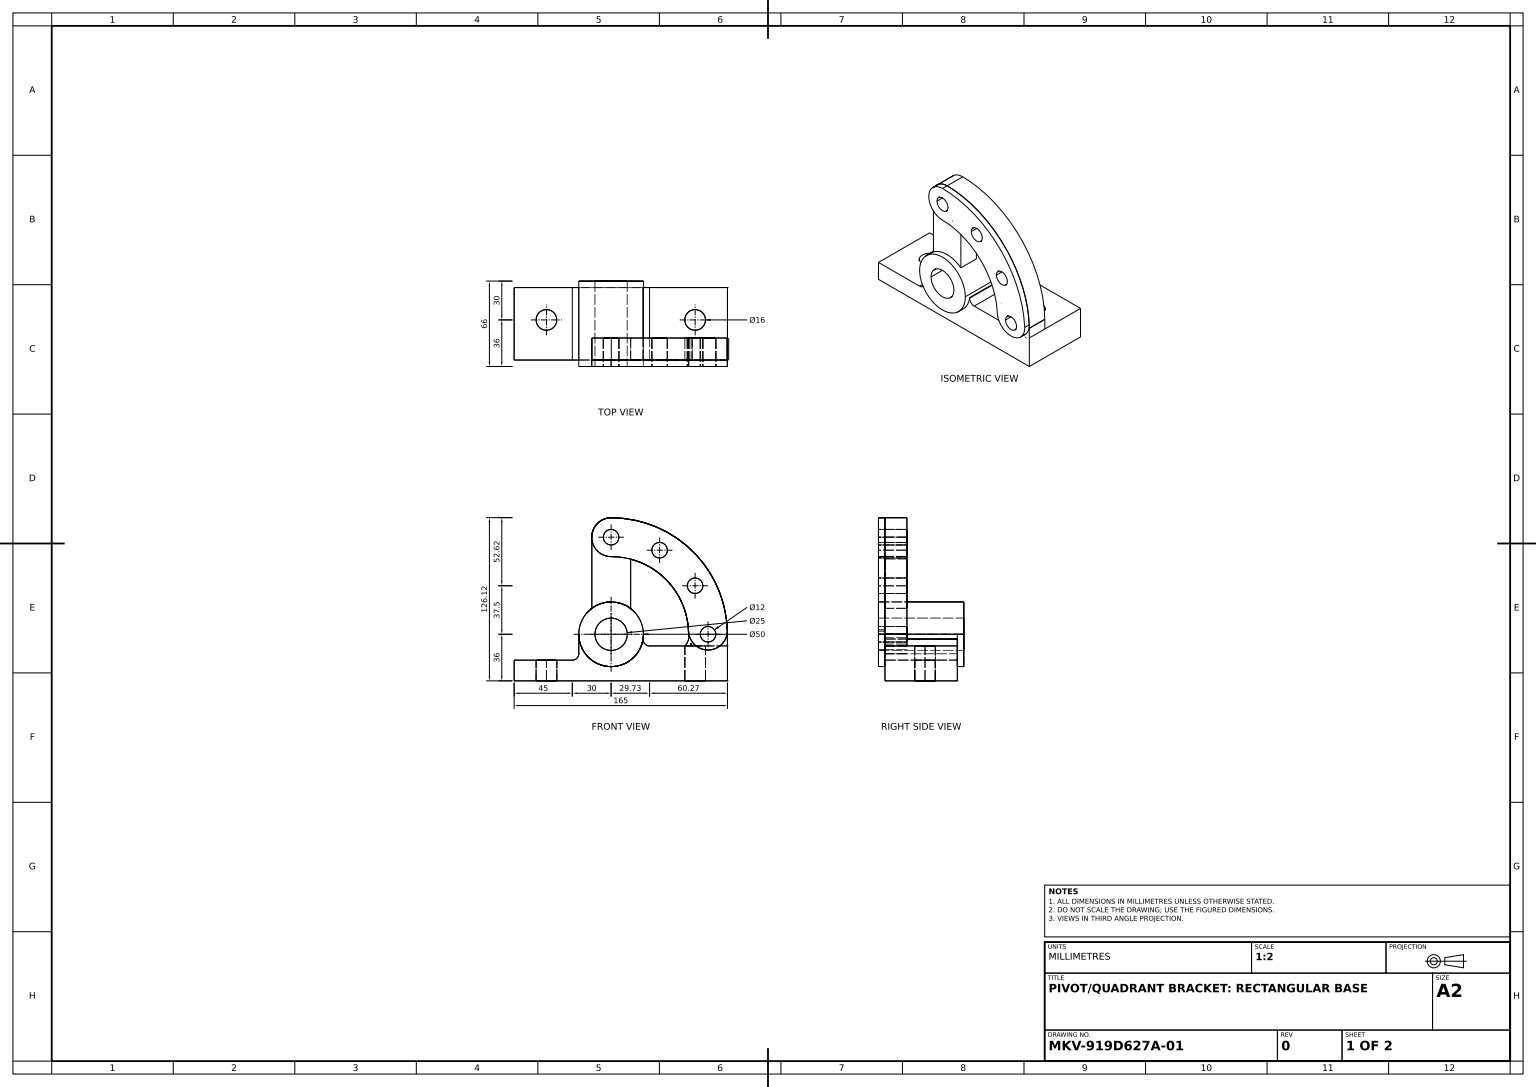
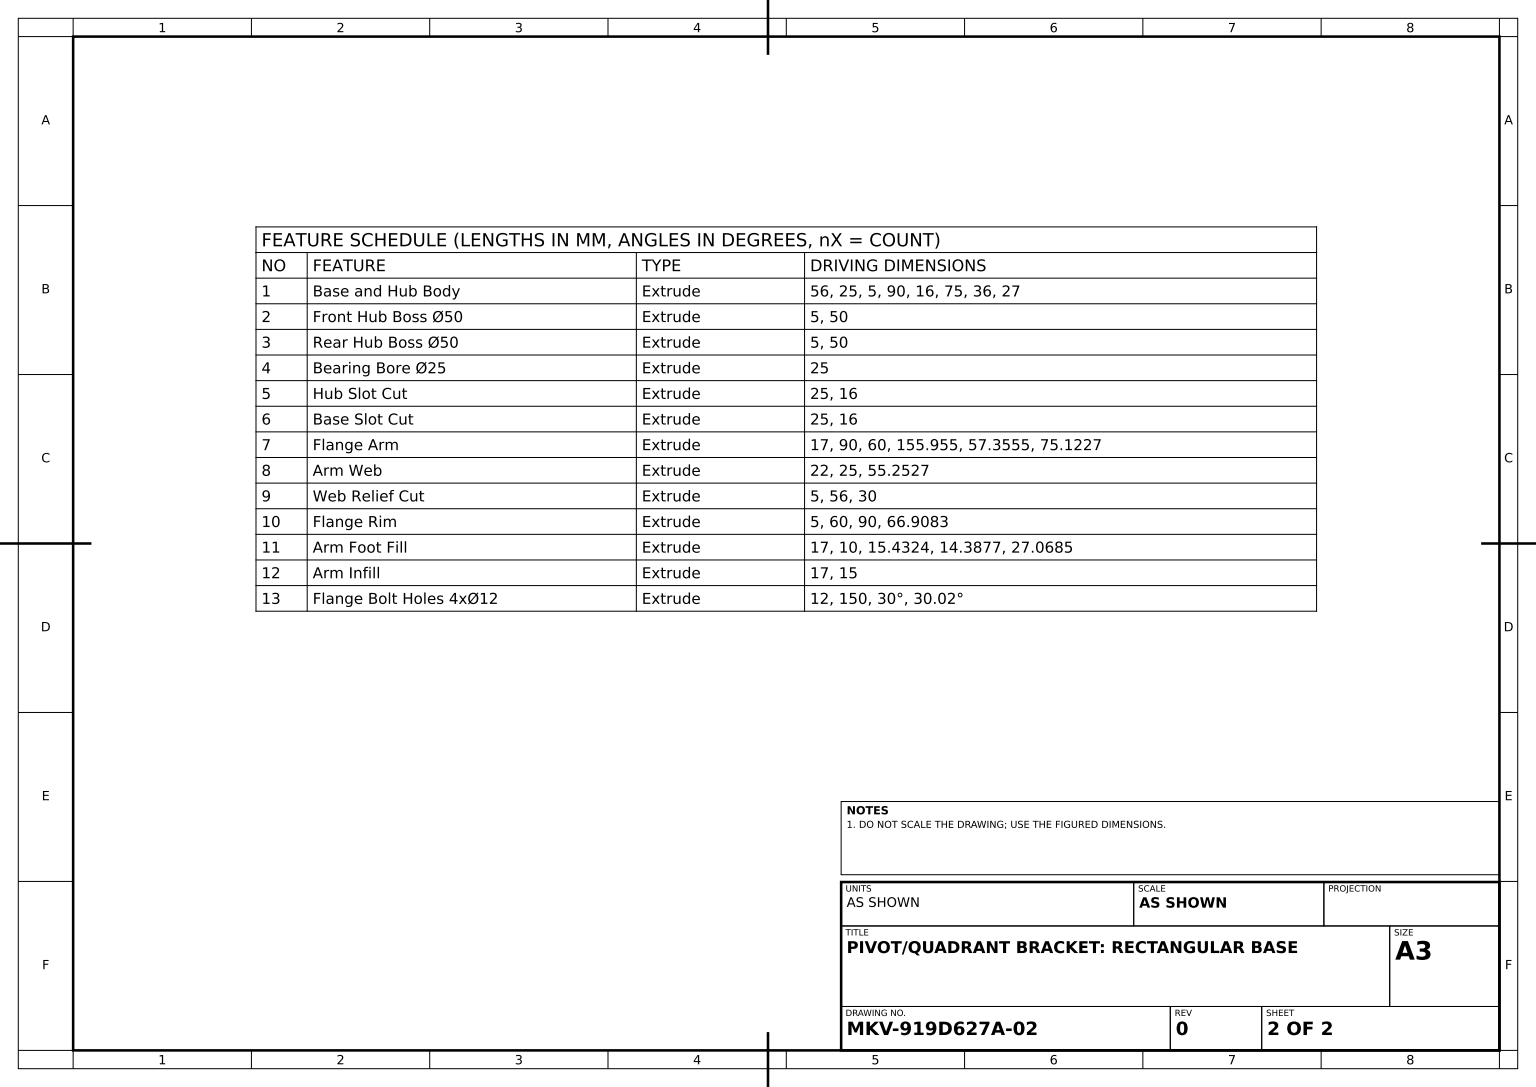
SolidWorks part; units mm, degrees
material "Plain Carbon Steel"
ref_plane "Front Plane" through (0, 0, 0) normal (0, 0, 1) x (1, 0, 0)
ref_plane "Top Plane" through (0, 0, 0) normal (0, 1, 0) x (1, 0, 0)
ref_plane "Right Plane" through (0, 0, 0) normal (1, 0, 0) x (0, 0, -1)
sketch "Base and Hub Profile Sketch" plane through (0, 0, 0) normal (0, 0, 1) x (1, 0, 0)
  line L0 (0, 0) -> (165, 0)
  line L1 (165, 0) -> (165, 27)
  line L2 (165, 27) -> (104.7321, 27)
  line L3 (0, 0) -> (0, 16)
  line L4 (0, 16) -> (45, 16)
  line L9 (50, 36) -> (50, 21)
  arc A0 (99.7768, 32.6667) -> (50, 36) centre (75, 36) ccw
  arc A1 (45, 16) -> (50, 21) centre (45, 21) ccw
  arc A2 (99.7768, 32.6667) -> (104.7321, 27) centre (104.7321, 32) ccw
  dimension "D1" = 75
  dimension "D2" = 25
  dimension "D4" = 5
  dimension "D8" = 5
  dimension "D3" = 36
  dimension "D5" = 90
  dimension "D6" = 16
  dimension "D7" = 27
extrude "Base and Hub Body" add sketch "Base and Hub Profile Sketch" along normal mid plane 56
sketch "Front Hub Boss Sketch" plane through (0, 0, 28) normal (0, 0, 1) x (1, 0, 0)
  circle A0 centre (75, 36) radius 25
  dimension "D1" = 50
extrude "Front Hub Boss Ø50" add sketch "Front Hub Boss Sketch" along normal blind 5
sketch "Rear Hub Boss Sketch" plane through (0, 0, -28) normal (0, 0, -1) x (-1, 0, 0)
  circle A0 centre (-75, 36) radius 25
  dimension "D1" = 50
extrude "Rear Hub Boss Ø50" add sketch "Rear Hub Boss Sketch" along normal blind 5
sketch "Bearing Bore Sketch" plane through (0, 0, 33) normal (0, 0, 1) x (1, 0, 0)
  circle A0 centre (75, 36) radius 12.5
  dimension "D1" = 25
extrude "Bearing Bore Ø25" cut sketch "Bearing Bore Sketch" against normal through all
sketch "Hub Slot Sketch" plane through (0, 16, 0) normal (0, 1, 0) x (1, 0, 0)
  line L0 (0, 28) -> (25, 28) construction
  line L1 (45, 28) -> (0, 28) construction
  line L2 (25, 28) -> (25, 3) construction
  line L3 (75, 33) -> (75, -33) construction
  line L4 (100, 33) -> (50, 33) construction
  line L5 (50, -33) -> (100, -33) construction
  circle A0 centre (25, 3) radius 8
  dimension "D1" = 25
  dimension "D3" = 16
  dimension "D2" = 25
extrude "Hub Slot Cut" cut sketch "Hub Slot Sketch" against normal through all
sketch "Base Slot Sketch" plane through (0, 27, 0) normal (0, 1, 0) x (1, 0, 0)
  line L0 (165, 28) -> (140, 28) construction
  line L1 (165, 28) -> (104.7321, 28) construction
  line L2 (140, 28) -> (140, 3) construction
  circle A0 centre (140, 3) radius 8
  dimension "D1" = 25
  dimension "D3" = 16
  dimension "D2" = 25
extrude "Base Slot Cut" cut sketch "Base Slot Sketch" against normal through all
sketch "Flange Arm Sketch" plane through (0, 0, 28) normal (0, 0, 1) x (1, 0, 0)
  line L0 (75, 36) -> (75.1126, 111.1227) construction
  line L1 (75, 36) -> (178.4698, 36) construction
  line L2 (75, 36) -> (128.0437, 89.0329) construction
  arc A0 (75.1126, 111.1227) -> (149.8877, 36) centre (74.8878, 36.1231) cw construction
  arc A1 (164.8877, 35.9754) -> (75.1576, 126.1227) centre (74.8878, 36.1231) ccw
  arc A2 (134.8877, 36.0246) -> (75.0677, 96.1228) centre (74.8878, 36.1231) ccw
  arc A3 (134.8877, 36.0246) -> (164.8877, 35.9754) centre (149.8877, 36) ccw
  arc A4 (75.1576, 126.1227) -> (75.0677, 96.1228) centre (75.1126, 111.1227) ccw
  point P6 (128.0437, 89.0329)
  dimension "D1" = 90
  dimension "D2" = 60
  dimension "D3" = 155.9553
  dimension "D4" = 57.3555
  dimension "D5" = 75.1227
extrude "Flange Arm" add sketch "Flange Arm Sketch" against normal blind 17
sketch "Arm Web Sketch" plane through (0, 0, 33) normal (0, 0, 1) x (1, 0, 0)
  line L0 (60.1127, 111.1677) -> (60.1127, 56.084)
  line L1 (60.1127, 111.1677) -> (90.1127, 111.1677)
  line L2 (90.1127, 111.1677) -> (90.1127, 55.915)
  line L3 (60.1127, 56.084) -> (90.1127, 55.915)
  arc A0 (75.1576, 126.1227) -> (75.0677, 96.1228) centre (75.1126, 111.1227) ccw construction
  circle A1 centre (75, 36) radius 25 construction
  arc A2 (90.1127, 55.915) -> (60.1127, 56.084) centre (75, 36) ccw
  circle M4 centre (75, 36) radius 25
  dimension "D1" = 55.2527
  dimension "D3" = 25
extrude "Arm Web" add sketch "Arm Web Sketch" against normal blind 22 contours L2 L1 L0 M4
sketch "Web Relief Sketch" plane through (0, 0, 33) normal (0, 0, 1) x (1, 0, 0)
  line L2 (60.1127, 56.084) -> (60.1127, 112.084)
  line L5 (60.1127, 112.084) -> (90.1127, 112.084)
  line L6 (90.1127, 112.084) -> (90.1127, 55.915)
  arc A1 (90.1127, 55.915) -> (60.1127, 56.084) centre (75, 36) ccw
  dimension "D1" = 56
  dimension "D3" = 30
extrude "Web Relief Cut" cut sketch "Web Relief Sketch" against normal blind 5
sketch "Flange Rim Sketch" plane through (0, 0, 28) normal (0, 0, 1) x (1, 0, 0)
  line L0 (60.1127, 111.0778) -> (60.1127, 56.084) construction
  arc A0 (149.9464, 38.8351) -> (75, 111) centre (75, 36) ccw construction
  arc A1 (164.9357, 39.4022) -> (75, 126) centre (75, 36) ccw
  arc A2 (134.9571, 38.2681) -> (75, 96) centre (75, 36) ccw
  arc A3 (134.9571, 38.2681) -> (164.9357, 39.4022) centre (149.9464, 38.8351) ccw
  arc A4 (75, 126) -> (75, 96) centre (75, 111) ccw
  point P4 (127.021, 90.0261)
  dimension "D1" = 60
  dimension "D2" = 90
  dimension "D3" = 66.9083
extrude "Flange Rim" add sketch "Flange Rim Sketch" along normal blind 5
sketch "Arm Foot Fill Sketch" plane through (0, 0, 28) normal (0, 0, 1) x (1, 0, 0)
  line L2 (132, 27) -> (137.8877, 27)
  arc A1 (135.096, 34.8587) -> (137.8192, 27) centre (150.5, 35.7953) ccw
  arc A3 (132, 27) -> (135.096, 34.8587) centre (125.1144, 34.2518) ccw
  arc M6 (134.8877, 36.0246) -> (137.8877, 27) centre (149.8877, 36) ccw
  dimension "D1" = 10
  dimension "D2" = 15.4324
  dimension "D3" = 14.3877
  dimension "D4" = 27.0685
extrude "Arm Foot Fill" add sketch "Arm Foot Fill Sketch" against normal blind 17 contours A3 L2 A1 M6
sketch "Arm Infill Sketch" plane through (0, 0, 28) normal (0, 0, 1) x (1, 0, 0)
  line L0 (161.8877, 27) -> (165, 27)
  line L2 (164.8877, 35.9754) -> (165, 27)
  arc A0 (164.8877, 35.9754) -> (161.8877, 27) centre (149.8877, 36) cw
  dimension "D1" = 15
extrude "Arm Infill" add sketch "Arm Infill Sketch" against normal blind 17
sketch "Flange Bolt Holes Sketch" plane through (0, 0, 33) normal (0, 0, 1) x (1, 0, 0)
  line L0 (75, 36) -> (164.8877, 35.9754) construction
  line L1 (75, 36) -> (139.9519, 73.5) construction
  line L2 (75, 36) -> (112.5, 100.9519) construction
  line L3 (75, 36) -> (75, 111) construction
  arc A0 (149.76, 30.0048) -> (69.0048, 110.76) centre (75, 36) ccw construction
  circle A1 centre (150, 36) radius 6
  circle A2 centre (75, 111) radius 6
  circle A3 centre (112.5, 100.9519) radius 6
  circle A4 centre (139.9519, 73.5) radius 6
  dimension "D1" = 12
  dimension "D2" = 150
  dimension "D5" = 12
  dimension "D6" = 12
  dimension "D7" = 12
  dimension "D3" = 30
  dimension "D4" = 30.016
extrude "Flange Bolt Holes 4xØ12" cut sketch "Flange Bolt Holes Sketch" against normal through all
